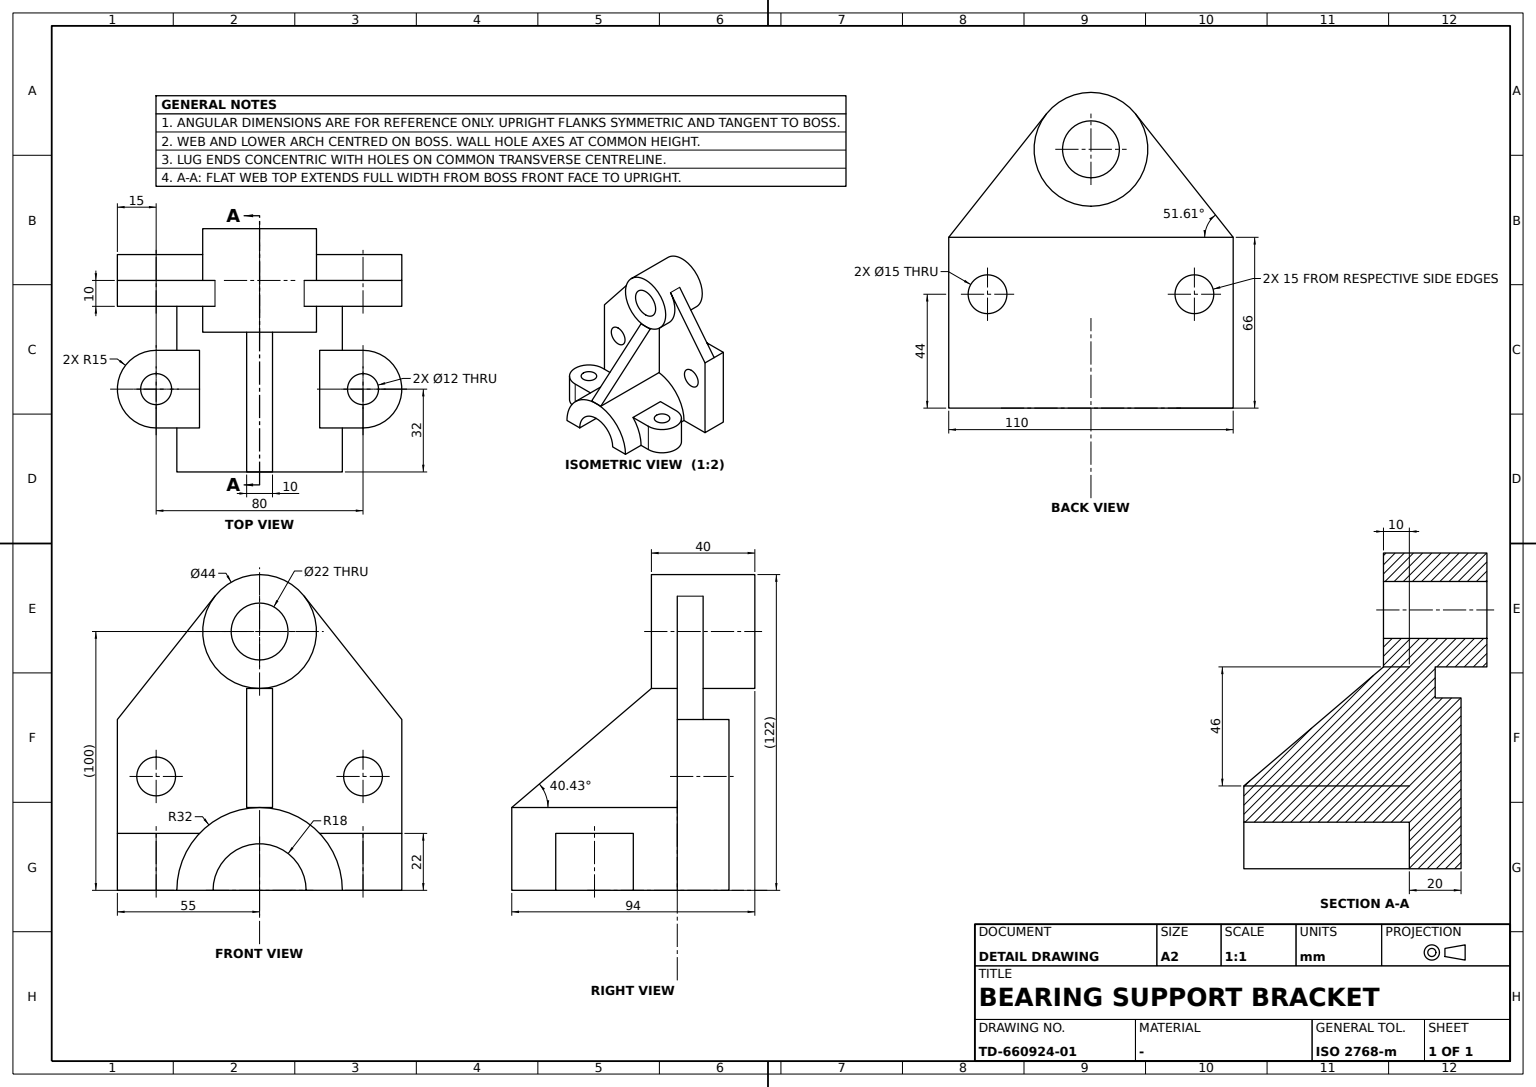
CATIA V5 part; units mm, degrees
sketch "Sketch1" plane through (0, 0, 0) normal (0, 1, 0) x (-1, 0, 0)
  arc A0 (32, 0) -> (-32, 0) centre (0, 0) ccw
  arc A1 (18, 0) -> (-18, 0) centre (0, 0) ccw
  line L0 (-32, 0) -> (-18, 0)
  point P0 (-32, 0)
  point P1 (18, 0)
  line L1 (18, 0) -> (32, 0)
  dimension "radius A0" = 32
  dimension "radius A1" = 18
  constraint coincidence P0 x-axis
  constraint coincidence L0 P1
  constraint coincidence L0 L1
  constraint horizontal L0 x-axis
  constraint horizontal L1 x-axis
extrude "Pad1" add sketch "Sketch1" along normal mid plane 64
sketch "Sketch2" plane through (0, -32, 0) normal (0, -1, 0) x (1, 0, 0)
  point P0 (55, 0)
  line L0 (55, 0) -> (55, 66)
  line L1 (55, 66) -> (-55, 66)
  line L2 (-55, 66) -> (-55, 0)
  point P1 (-55, 0)
  line L3 (-55, 0) -> (55, 0)
  dimension "length L0" = 66
  dimension "length L3" = 110
  constraint coincidence P0 x-axis
  constraint coincidence P1 x-axis
  constraint vertical L0 y-axis
  constraint vertical L2 y-axis
  constraint horizontal L1 x-axis
  constraint horizontal L3 x-axis
  constraint symmetry L0 L2 y-axis
extrude "Pad2" add sketch "Sketch2" along normal blind 20
sketch "Sketch3" plane through (0, -32, 0) normal (0, 1, 0) x (-1, 0, 0)
  arc A0 (-17.2448, 113.6607) -> (17.2448, 113.6607) centre (0, 100) ccw
  point P0 (0, 100)
  line L0 (-17.2448, 113.6607) -> (-55, 66)
  point P1 (-55, 66)
  line L1 (-55, 66) -> (55, 66)
  point P2 (55, 66)
  line L2 (55, 66) -> (17.2448, 113.6607)
  line L3 (-55, 66) -> (55, 66) construction
  point P3 (-55, 66)
  line L4 (55, 66) -> (55, 0) construction
  line L5 (55, 0) -> (-55, 0) construction
  dimension "radius A0" = 22
  dimension "distance P0 L5" = 100
  constraint coincidence P0 y-axis
  constraint coincidence L1 L3
  constraint coincidence P1 P3
  constraint coincidence P2 L4
  constraint horizontal L1 x-axis
  constraint tangency L0 A0
  constraint tangency L2 A0
extrude "Pad3" add sketch "Sketch3" against normal blind 10
sketch "Sketch4" plane through (0, -42, 0) normal (0, -1, 0) x (1, 0, 0)
  circle A0 centre (0, 100) radius 22
  point P0 (0, 100)
  point P1 (0, 78)
  circle A1 centre (0, 100) radius 11
  dimension "radius A1" = 11
  dimension "radius A0" = 22
  dimension "distance P0 x axis" = 100
  constraint coincidence P0 y-axis
  constraint coincidence A0 P1
  constraint coincidence P1 y-axis
extrude "Pad4" add sketch "Sketch4" along normal mid plane 40
sketch "Sketch5" plane through (0, 0, 0) normal (0, 0, 1) x (0, 1, 0)
  arc A0 (-15, -40) -> (15, -40) centre (0, -40) ccw
  point P0 (0, -55)
  circle A1 centre (0, -40) radius 6
  point P1 (-15, -40)
  line L0 (-15, -20) -> (15, -20)
  line L1 (15, -20) -> (15, -40)
  point P2 (15, -40)
  line L2 (-15, -40) -> (-15, -20)
  point P3 (-15, -40)
  point P4 (15, -40)
  dimension "radius A1" = 6
  dimension "radius A0" = 15
  dimension "length L1" = 20
  dimension "distance x axis P2" = 40
  constraint coincidence A0 P0
  constraint coincidence P0 y-axis
  constraint coincidence P1 A0
  constraint coincidence P2 P4
  constraint coincidence P1 P3
  constraint horizontal L0 x-axis
  constraint tangency L1 A0
  constraint tangency L2 A0
  constraint vertical L1 y-axis
  constraint vertical L2 y-axis
  constraint symmetry L1 L2 y-axis
  constraint concentricity A0 A1
extrude "Pad5" add sketch "Sketch5" along normal blind 22
mirror "Mirror1" about plane through (0, 0, 0) normal (1, 0, 0) of "Pad5"
sketch "Sketch6" plane through (36.0539, -32, 61.7346) normal (0, 1, 0) x (1, 0, 0)
  point P0 (3.9461, 17.7346)
  line L0 (-91.0539, 61.7346) -> (18.9461, 61.7346) construction
  dimension "distance P0 L0" = 44
  dimension "D2" = 40
hole "Hole1" at (40, -32, 44) direction (0, -1, 0) diameter 15 end through all
mirror "Mirror2" about plane through (0, 0, 0) normal (1, 0, 0) of "Hole1"
sketch "Sketch7" plane through (0, 0, 0) normal (1, 0, 0) x (0, 1, 0)
  point P0 (-22, 78)
  line L0 (-22, 78) -> (32, 32)
  point P1 (32, 32)
  point P2 (-22, 78)
  line L1 (-22, 78) -> (-32, 78)
  line L2 (-32, 78) -> (-32, 32)
  line L3 (-32, 32) -> (32, 32)
  line L4 (-32, 0) -> (-32, 66) construction
  line L5 (32, 32) -> (32, 0) construction
  dimension "D1" = 32
  dimension "length L2" = 46
  dimension "length L1" = 10
  constraint coincidence P2 L0
  constraint coincidence L2 L4
  constraint coincidence P1 L5
  constraint coincidence P0 P2
  constraint horizontal L1 x-axis
  constraint horizontal L3 x-axis
  constraint vertical L2 y-axis
extrude "Pad6" add sketch "Sketch7" along normal mid plane 10
